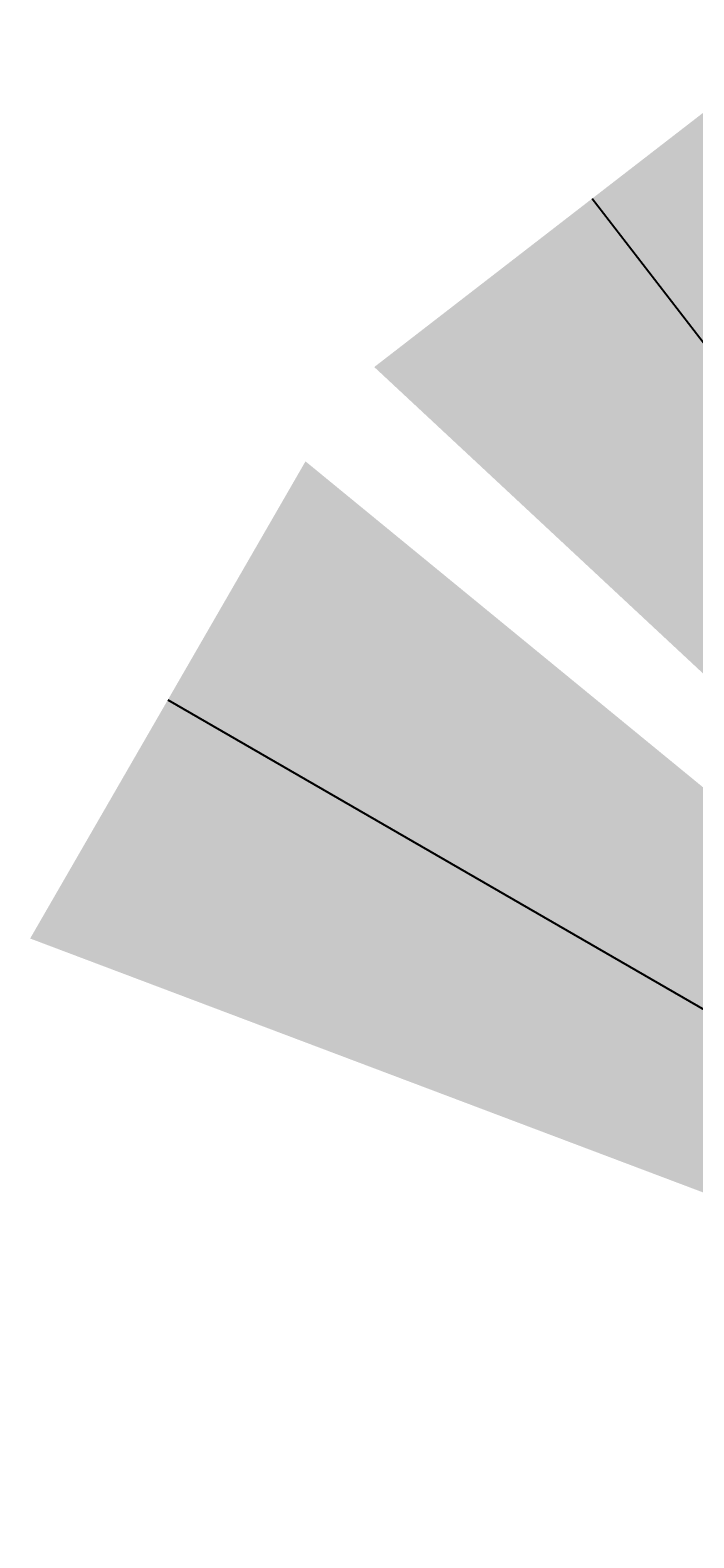
# Model space of a CAD drawing. Units: inches. Extents: x -9413 to 9703, y -9719 to 9096.
# Tile 1 of 1: x -9413 to -5451, y 99 to 9096. Entities that reach past the tile are written whole.
import ezdxf
from ezdxf import colors
from ezdxf.entities.mleader import LeaderData, LeaderLine
from ezdxf.math import Vec2, Vec3

# ---------------------------------------------------------------- set-up
doc = ezdxf.new("R2010")
doc.units = ezdxf.units.IN
doc.header["$MEASUREMENT"] = 0
doc.layers.add('M-ANNO-TEXT', color=7, linetype='Continuous', lineweight=18)
doc.styles.get("Standard").update_dxf_attribs({"font": 'arial.ttf'})

msp = doc.modelspace()

# ---------------------------------------------------------------- leaders
at = {"layer": 'M-ANNO-TEXT'}
ml = msp.add_multileader_mtext('Standard', dxfattribs=at)
ml.set_content('steam drum', color=256)
ml.set_leader_properties()
ml.build(insert=Vec2(0, 0))
ml.multileader.update_dxf_attribs({"dogleg_length": 0.36, "arrow_head_size": 10000, "scale": 10})
ctx = ml.context
ctx.base_point, ctx.scale, ctx.char_height, ctx.arrow_head_size, ctx.landing_gap_size, ctx.plane_origin = Vec3(1.078100315116472, 187.1657656808087), 10, 5.4, 10000, 0.9, Vec3(56.53630785249729, 178.1917761520126)
ctx.text_align_type = 2
notes = []
notes.append((ctx, [(0, (1, 1, 0), (49.60206616053652, 187.1657656808087), (-1, 0), 7.616326009130828, [(0, [(56.5363078524973, 178.1917761520126)], 0, [])])]))
ctx.mtext.insert, ctx.mtext.alignment, ctx.mtext.flow_direction = Vec3(41.08574015140569, 189.9099675907678), 3, 5
ml = msp.add_multileader_mtext('Standard', dxfattribs=at)
ml.set_content('Boiler', color=256)
ml.set_leader_properties()
ml.build(insert=Vec2(0, 0))
ml.multileader.update_dxf_attribs({"dogleg_length": 0.36, "arrow_head_size": 10000, "scale": 10})
ctx = ml.context
ctx.base_point, ctx.scale, ctx.char_height, ctx.arrow_head_size, ctx.landing_gap_size, ctx.plane_origin = Vec3(31.04430257849453, 103.0991380116177), 10, 5.4, 10000, 0.9, Vec3(69.11352005531556, 99.3051261342938)
ctx.text_align_type = 2
notes.append((ctx, [(0, (1, 1, 0), (62.54209871927075, 103.0991380116177), (-1, 0), 10.86041551321825, [(0, [(69.11352005531556, 99.3051261342938)], 0, [])])]))
ctx.mtext.insert, ctx.mtext.alignment, ctx.mtext.flow_direction = Vec3(50.7816832060525, 105.8433399215768), 3, 5
for ctx, leaders in notes:
    for number, flags, end, landing, length, lines in leaders:
        leader = LeaderData()
        leader.index, (leader.has_last_leader_line, leader.has_dogleg_vector, leader.attachment_direction) = number, flags
        leader.last_leader_point, leader.dogleg_vector, leader.dogleg_length = Vec3(end), Vec3(landing), length
        for number, points, colour, breaks in lines:
            line = LeaderLine()
            line.index, line.vertices, line.color, line.breaks = number, Vec3.list(points), colors.encode_raw_color(colour), breaks
            leader.lines.append(line)
        ctx.leaders.append(leader)

doc.saveas('drawing.dxf')
